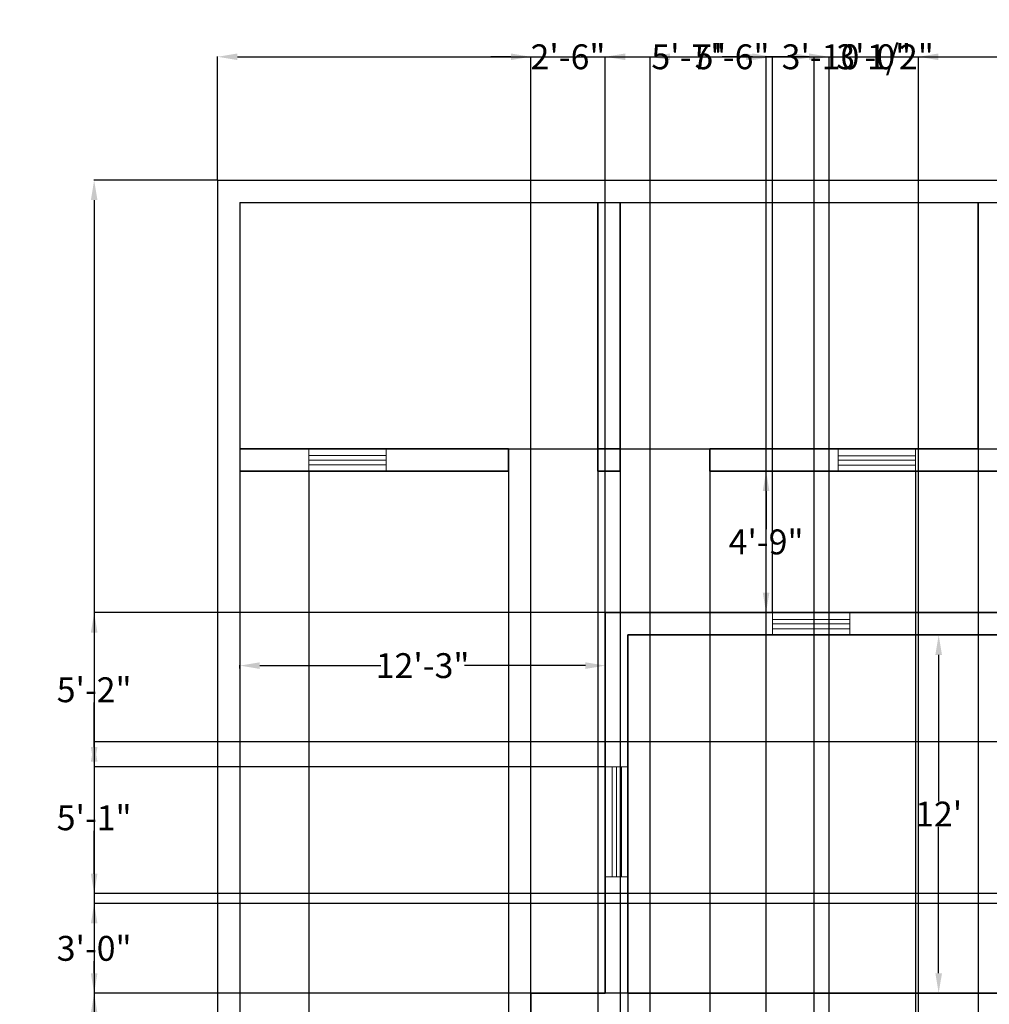
# Model space of a CAD drawing. Units: inches. Extents: x -63 to 800, y 3068 to 4133.
# Tile 4 of 5: x -63 to 327, y 3737 to 4133. Entities that reach past the tile are written whole.
import ezdxf

# ---------------------------------------------------------------- set-up
doc = ezdxf.new("R2010")
doc.units = ezdxf.units.IN
doc.header["$MEASUREMENT"] = 0
for name, color, linetype, lineweight in [('A-ANNO-DIMS', 2, 'Continuous', 13), ('A-GLAZ', 4, 'Continuous', 18), ('A-WALL', 7, 'Continuous', 35), ('A-WALL-SITE', 8, 'Continuous', 30)]:
    doc.layers.add(name, color=color, linetype=linetype, lineweight=lineweight)
doc.styles.get("Standard").update_dxf_attribs({"font": 'arial.ttf'})
doc.dimstyles.get("Standard").update_dxf_attribs({"dimtxt": 10, "dimasz": 8, "dimexe": 0.18, "dimexo": 0.0625, "dimgap": 0.09, "dimtad": 0, "dimtih": 1, "dimtoh": 1, "dimdec": 0, "dimzin": 0, "dimdsep": 46, "dimlunit": 3, "dimtxsty": 'Standard', "dimcen": 0.09, "dimadec": 0, "dimazin": 0, "dimtfac": 1, "dimtdec": 0, "dimtofl": 0, "dimtmove": 0, "dimatfit": 3, "dimfxl": 1, "dimtolj": 1, "dimtzin": 0, "dimarcsym": 0})

# ---------------------------------------------------------------- blocks, each defined once
blk = doc.blocks.new('*D2')
at = {"layer": 'A-ANNO-DIMS', "color": 0, "lineweight": -2, "transparency": 16777216}
for p, q in [((223.3, 3951.66), (237.18, 3951.66)), ((237, 3943.66), (237, 3928.43)), ((237, 3902.81), (237, 3918.04)), ((223.3, 3894.81), (237.18, 3894.81))]:
    blk.add_line(p, q, dxfattribs=at)
at = {"layer": 'A-ANNO-DIMS', "color": 0, "transparency": 16777216}
for points in [[(235.66, 3943.66), (238.33, 3943.66), (237, 3951.66)], [(235.66, 3902.81), (238.33, 3902.81), (237, 3894.81)]]:
    blk.add_solid(points, dxfattribs=at)
at = {"layer": 'Defpoints', "color": 0, "transparency": 16777216}
for p in [(223.24, 3951.66), (223.24, 3894.81), (237, 3894.81)]:
    blk.add_point(p, dxfattribs=at)
at = {"layer": 'A-ANNO-DIMS', "color": 0, "transparency": 16777216, "insert": (237, 3923.24), "char_height": 10, "attachment_point": 5}
blk.add_mtext('\\A1;4\'-9"', dxfattribs=at)
blk = doc.blocks.new('*D3')
at = {"layer": 'A-ANNO-DIMS', "color": 0, "lineweight": -2, "transparency": 16777216}
for p, q in [((25.31, 3872.29), (25.31, 3873.68)), ((33.31, 3873.5), (82.01, 3873.5)), ((164.31, 3873.5), (115.6, 3873.5)), ((172.31, 3872.29), (172.31, 3873.68))]:
    blk.add_line(p, q, dxfattribs=at)
at = {"layer": 'A-ANNO-DIMS', "color": 0, "transparency": 16777216}
for points in [[(33.31, 3874.83), (33.31, 3872.16), (25.31, 3873.5)], [(164.31, 3874.83), (164.31, 3872.16), (172.31, 3873.5)]]:
    blk.add_solid(points, dxfattribs=at)
at = {"layer": 'Defpoints', "color": 0, "transparency": 16777216}
for p in [(25.31, 3872.23), (172.31, 3873.5), (172.31, 3872.23)]:
    blk.add_point(p, dxfattribs=at)
at = {"layer": 'A-ANNO-DIMS', "color": 0, "transparency": 16777216, "insert": (98.81, 3873.5), "char_height": 10, "attachment_point": 5}
blk.add_mtext('\\A1;12\'-3"', dxfattribs=at)
blk = doc.blocks.new('*D5')
at = {"layer": 'A-ANNO-DIMS', "color": 0, "lineweight": -2, "transparency": 16777216}
for p, q in [((306.49, 3885.81), (306.61, 3885.81)), ((306.43, 3877.81), (306.43, 3818.92)), ((306.43, 3749.81), (306.43, 3808.7)), ((306.49, 3741.81), (306.61, 3741.81))]:
    blk.add_line(p, q, dxfattribs=at)
at = {"layer": 'A-ANNO-DIMS', "color": 0, "transparency": 16777216}
for points in [[(305.1, 3877.81), (307.77, 3877.81), (306.43, 3885.81)], [(305.1, 3749.81), (307.77, 3749.81), (306.43, 3741.81)]]:
    blk.add_solid(points, dxfattribs=at)
at = {"layer": 'Defpoints', "color": 0, "transparency": 16777216}
for p in [(306.43, 3885.81), (306.43, 3741.81), (306.43, 3741.81)]:
    blk.add_point(p, dxfattribs=at)
at = {"layer": 'A-ANNO-DIMS', "color": 0, "transparency": 16777216, "insert": (306.43, 3813.81), "char_height": 10, "attachment_point": 5}
blk.add_mtext("\\A1;12'", dxfattribs=at)
blk = doc.blocks.new('WIN-31')
blk.add_lwpolyline([(0, 9), (31.17, 9), (31.17, 0), (0, 0)], close=True)
blk.add_lwpolyline([(0, 4.5), (31.17, 4.5), (31.17, 6.29), (0, 6.29), (0, 2.51), (31.17, 2.51)])
blk = doc.blocks.new('WIN-44')
blk.add_lwpolyline([(0, 0), (0, 44.17), (9, 44.17), (9, 0)], close=True)
for points in [[(2.71, 44.17), (2.71, 0), (6.5, 0), (6.5, 44.17)], [(4.5, 0), (4.5, 44.17)]]:
    blk.add_lwpolyline(points)
blk = doc.blocks.new('*D19')
at = {"layer": 'A-ANNO-DIMS', "color": 0, "lineweight": -2, "transparency": 16777216}
for p, q in [((16.31, 4068.72), (16.31, 4118.49)), ((24.31, 4118.31), (351.54, 4118.31)), ((713.31, 4118.31), (386.08, 4118.31)), ((721.31, 4068.72), (721.31, 4118.49))]:
    blk.add_line(p, q, dxfattribs=at)
at = {"layer": 'A-ANNO-DIMS', "color": 0, "transparency": 16777216}
for points in [[(24.31, 4119.64), (24.31, 4116.98), (16.31, 4118.31)], [(713.31, 4119.64), (713.31, 4116.98), (721.31, 4118.31)]]:
    blk.add_solid(points, dxfattribs=at)
at = {"layer": 'Defpoints', "color": 0, "transparency": 16777216}
for p in [(721.31, 4118.31), (16.31, 4068.66), (721.31, 4068.66)]:
    blk.add_point(p, dxfattribs=at)
at = {"layer": 'A-ANNO-DIMS', "color": 0, "transparency": 16777216, "insert": (368.81, 4118.31), "char_height": 10, "attachment_point": 5}
blk.add_mtext('\\A1;58\'-9"', dxfattribs=at)
blk = doc.blocks.new('*D20')
at = {"layer": 'A-ANNO-DIMS', "color": 0, "lineweight": -2, "transparency": 16777216}
for p, q in [((16.25, 4068.66), (-33.52, 4068.66)), ((-33.34, 4060.66), (-33.34, 3605.75)), ((-33.34, 3140.31), (-33.34, 3595.23)), ((16.25, 3132.31), (-33.52, 3132.31))]:
    blk.add_line(p, q, dxfattribs=at)
at = {"layer": 'A-ANNO-DIMS', "color": 0, "transparency": 16777216}
for points in [[(-34.67, 4060.66), (-32.01, 4060.66), (-33.34, 4068.66)], [(-34.67, 3140.31), (-32.01, 3140.31), (-33.34, 3132.31)]]:
    blk.add_solid(points, dxfattribs=at)
at = {"layer": 'Defpoints', "color": 0, "transparency": 16777216}
for p in [(-33.34, 4068.66), (16.31, 4068.66), (16.31, 3132.31)]:
    blk.add_point(p, dxfattribs=at)
at = {"layer": 'A-ANNO-DIMS', "color": 0, "transparency": 16777216, "insert": (-33.34, 3600.49), "char_height": 10, "attachment_point": 5}
blk.add_mtext('\\A1;78\'-0 1/2"', dxfattribs=at)
blk = doc.blocks.new('*D23')
at = {"layer": 'A-ANNO-DIMS', "color": 0, "lineweight": -2, "transparency": 16777216}
for p, q in [((25.31, 4059.6), (25.31, 3082.48)), ((169.31, 4059.6), (169.31, 3082.48)), ((33.31, 3082.66), (80.51, 3082.66)), ((161.31, 3082.66), (114.1, 3082.66))]:
    blk.add_line(p, q, dxfattribs=at)
at = {"layer": 'A-ANNO-DIMS', "color": 0, "transparency": 16777216}
for points in [[(33.31, 3083.99), (33.31, 3081.33), (25.31, 3082.66)], [(161.31, 3083.99), (161.31, 3081.33), (169.31, 3082.66)]]:
    blk.add_solid(points, dxfattribs=at)
at = {"layer": 'Defpoints', "color": 0, "transparency": 16777216}
for p in [(25.31, 4059.66), (169.31, 4059.66), (169.31, 3082.66)]:
    blk.add_point(p, dxfattribs=at)
at = {"layer": 'A-ANNO-DIMS', "color": 0, "transparency": 16777216, "insert": (97.31, 3082.66), "char_height": 10, "attachment_point": 5}
blk.add_mtext('\\A1;12\'-0"', dxfattribs=at)
blk = doc.blocks.new('*D24')
at = {"layer": 'A-ANNO-DIMS', "color": 0, "lineweight": -2, "transparency": 16777216}
for p, q in [((178.31, 4059.6), (178.31, 3082.48)), ((322.31, 4059.6), (322.31, 3082.48)), ((186.31, 3082.66), (233.51, 3082.66)), ((314.31, 3082.66), (267.1, 3082.66))]:
    blk.add_line(p, q, dxfattribs=at)
at = {"layer": 'A-ANNO-DIMS', "color": 0, "transparency": 16777216}
for points in [[(186.31, 3083.99), (186.31, 3081.33), (178.31, 3082.66)], [(314.31, 3083.99), (314.31, 3081.33), (322.31, 3082.66)]]:
    blk.add_solid(points, dxfattribs=at)
at = {"layer": 'Defpoints', "color": 0, "transparency": 16777216}
for p in [(178.31, 4059.66), (322.31, 4059.66), (322.31, 3082.66)]:
    blk.add_point(p, dxfattribs=at)
at = {"layer": 'A-ANNO-DIMS', "color": 0, "transparency": 16777216, "insert": (250.31, 3082.66), "char_height": 10, "attachment_point": 5}
blk.add_mtext('\\A1;12\'-0"', dxfattribs=at)
blk = doc.blocks.new('*D26')
at = {"layer": 'A-ANNO-DIMS', "color": 0, "lineweight": -2, "transparency": 16777216}
for p, q in [((25.37, 4059.66), (771.14, 4059.66)), ((770.96, 4051.66), (770.96, 4015.36)), ((770.96, 3968.66), (770.96, 4004.96)), ((25.37, 3960.66), (771.14, 3960.66))]:
    blk.add_line(p, q, dxfattribs=at)
at = {"layer": 'A-ANNO-DIMS', "color": 0, "transparency": 16777216}
for points in [[(769.63, 4051.66), (772.29, 4051.66), (770.96, 4059.66)], [(769.63, 3968.66), (772.29, 3968.66), (770.96, 3960.66)]]:
    blk.add_solid(points, dxfattribs=at)
at = {"layer": 'Defpoints', "color": 0, "transparency": 16777216}
for p in [(25.31, 4059.66), (770.96, 4059.66), (25.31, 3960.66)]:
    blk.add_point(p, dxfattribs=at)
at = {"layer": 'A-ANNO-DIMS', "color": 0, "transparency": 16777216, "insert": (770.96, 4010.16), "char_height": 10, "attachment_point": 5}
blk.add_mtext('\\A1;8\'-3"', dxfattribs=at)
blk = doc.blocks.new('*D27')
at = {"layer": 'A-ANNO-DIMS', "color": 0, "lineweight": -2, "transparency": 16777216}
for p, q in [((25.31, 3951.6), (25.31, 3082.48)), ((52.97, 3951.6), (52.97, 3082.48)), ((33.31, 3082.66), (44.97, 3082.66)), ((52.97, 3082.66), (60.97, 3082.66))]:
    blk.add_line(p, q, dxfattribs=at)
at = {"layer": 'A-ANNO-DIMS', "color": 0, "transparency": 16777216}
for points in [[(33.31, 3083.99), (33.31, 3081.33), (25.31, 3082.66)], [(44.97, 3083.99), (44.97, 3081.33), (52.97, 3082.66)]]:
    blk.add_solid(points, dxfattribs=at)
at = {"layer": 'Defpoints', "color": 0, "transparency": 16777216}
for p in [(25.31, 3951.66), (52.97, 3951.66), (52.97, 3082.66)]:
    blk.add_point(p, dxfattribs=at)
at = {"layer": 'A-ANNO-DIMS', "color": 0, "transparency": 16777216, "insert": (86.08, 3082.66), "char_height": 10, "attachment_point": 5}
blk.add_mtext('\\A1;2\'-3 1/2"', dxfattribs=at)
blk = doc.blocks.new('*D28')
at = {"layer": 'A-ANNO-DIMS', "color": 0, "lineweight": -2, "transparency": 16777216}
for p, q in [((297.16, 3951.55), (297.16, 3082.48)), ((331.31, 3951.6), (331.31, 3082.48)), ((305.16, 3082.66), (323.31, 3082.66)), ((331.31, 3082.66), (339.31, 3082.66))]:
    blk.add_line(p, q, dxfattribs=at)
at = {"layer": 'A-ANNO-DIMS', "color": 0, "transparency": 16777216}
for points in [[(305.16, 3083.99), (305.16, 3081.33), (297.16, 3082.66)], [(323.31, 3083.99), (323.31, 3081.33), (331.31, 3082.66)]]:
    blk.add_solid(points, dxfattribs=at)
at = {"layer": 'Defpoints', "color": 0, "transparency": 16777216}
for p in [(297.16, 3951.61), (331.31, 3951.66), (331.31, 3082.66)]:
    blk.add_point(p, dxfattribs=at)
at = {"layer": 'A-ANNO-DIMS', "color": 0, "transparency": 16777216, "insert": (356.66, 3082.66), "char_height": 10, "attachment_point": 5}
blk.add_mtext('\\A1;2\'-10"', dxfattribs=at)
blk = doc.blocks.new('*D30')
at = {"layer": 'A-ANNO-DIMS', "color": 0, "lineweight": -2, "transparency": 16777216}
for p, q in [((133.31, 3951.6), (133.31, 3082.48)), ((169.31, 3951.6), (169.31, 3082.48)), ((125.31, 3082.66), (117.31, 3082.66)), ((177.31, 3082.66), (185.31, 3082.66))]:
    blk.add_line(p, q, dxfattribs=at)
at = {"layer": 'A-ANNO-DIMS', "color": 0, "transparency": 16777216}
for points in [[(125.31, 3083.99), (125.31, 3081.33), (133.31, 3082.66)], [(177.31, 3083.99), (177.31, 3081.33), (169.31, 3082.66)]]:
    blk.add_solid(points, dxfattribs=at)
at = {"layer": 'Defpoints', "color": 0, "transparency": 16777216}
for p in [(133.31, 3951.66), (169.31, 3951.66), (169.31, 3082.66)]:
    blk.add_point(p, dxfattribs=at)
at = {"layer": 'A-ANNO-DIMS', "color": 0, "transparency": 16777216, "insert": (151.31, 3082.66), "char_height": 10, "attachment_point": 5}
blk.add_mtext('\\A1;3\'-0"', dxfattribs=at)
blk = doc.blocks.new('*D31')
at = {"layer": 'A-ANNO-DIMS', "color": 0, "lineweight": -2, "transparency": 16777216}
for p, q in [((178.31, 3951.6), (178.31, 3082.48)), ((214.31, 3951.6), (214.31, 3082.48)), ((170.31, 3082.66), (162.31, 3082.66)), ((222.31, 3082.66), (230.31, 3082.66))]:
    blk.add_line(p, q, dxfattribs=at)
at = {"layer": 'A-ANNO-DIMS', "color": 0, "transparency": 16777216}
for points in [[(170.31, 3083.99), (170.31, 3081.33), (178.31, 3082.66)], [(222.31, 3083.99), (222.31, 3081.33), (214.31, 3082.66)]]:
    blk.add_solid(points, dxfattribs=at)
at = {"layer": 'Defpoints', "color": 0, "transparency": 16777216}
for p in [(178.31, 3951.66), (214.31, 3951.66), (214.31, 3082.66)]:
    blk.add_point(p, dxfattribs=at)
at = {"layer": 'A-ANNO-DIMS', "color": 0, "transparency": 16777216, "insert": (196.31, 3082.66), "char_height": 10, "attachment_point": 5}
blk.add_mtext('\\A1;3\'-0"', dxfattribs=at)
blk = doc.blocks.new('*D32')
at = {"layer": 'A-ANNO-DIMS', "color": 0, "lineweight": -2, "transparency": 16777216}
for p, q in [((331.31, 3951.6), (331.31, 3082.48)), ((367.31, 3951.6), (367.31, 3082.48)), ((323.31, 3082.66), (315.31, 3082.66)), ((375.31, 3082.66), (383.31, 3082.66))]:
    blk.add_line(p, q, dxfattribs=at)
at = {"layer": 'A-ANNO-DIMS', "color": 0, "transparency": 16777216}
for points in [[(323.31, 3083.99), (323.31, 3081.33), (331.31, 3082.66)], [(375.31, 3083.99), (375.31, 3081.33), (367.31, 3082.66)]]:
    blk.add_solid(points, dxfattribs=at)
at = {"layer": 'Defpoints', "color": 0, "transparency": 16777216}
for p in [(331.31, 3951.66), (367.31, 3951.66), (367.31, 3082.66)]:
    blk.add_point(p, dxfattribs=at)
at = {"layer": 'A-ANNO-DIMS', "color": 0, "transparency": 16777216, "insert": (349.31, 3082.66), "char_height": 10, "attachment_point": 5}
blk.add_mtext('\\A1;3\'-0"', dxfattribs=at)
blk = doc.blocks.new('*D36')
at = {"layer": 'A-ANNO-DIMS', "color": 0, "lineweight": -2, "transparency": 16777216}
for p, q in [((134.31, 4118.31), (126.31, 4118.31)), ((142.31, 3741.87), (142.31, 4118.49)), ((172.31, 3741.87), (172.31, 4118.49)), ((180.31, 4118.31), (188.31, 4118.31))]:
    blk.add_line(p, q, dxfattribs=at)
at = {"layer": 'A-ANNO-DIMS', "color": 0, "transparency": 16777216}
for points in [[(134.31, 4119.64), (134.31, 4116.98), (142.31, 4118.31)], [(180.31, 4119.64), (180.31, 4116.98), (172.31, 4118.31)]]:
    blk.add_solid(points, dxfattribs=at)
at = {"layer": 'Defpoints', "color": 0, "transparency": 16777216}
for p in [(172.31, 4118.31), (142.31, 3741.81), (172.31, 3741.81)]:
    blk.add_point(p, dxfattribs=at)
at = {"layer": 'A-ANNO-DIMS', "color": 0, "transparency": 16777216, "insert": (157.31, 4118.31), "char_height": 10, "attachment_point": 5}
blk.add_mtext('\\A1;2\'-6"', dxfattribs=at)
blk = doc.blocks.new('*D37')
at = {"layer": 'A-ANNO-DIMS', "color": 0, "lineweight": -2, "transparency": 16777216}
for p, q in [((181.31, 3885.75), (181.31, 3082.48)), ((349.31, 3885.75), (349.31, 3082.48)), ((189.31, 3082.66), (248.51, 3082.66)), ((341.31, 3082.66), (282.1, 3082.66))]:
    blk.add_line(p, q, dxfattribs=at)
at = {"layer": 'A-ANNO-DIMS', "color": 0, "transparency": 16777216}
for points in [[(189.31, 3083.99), (189.31, 3081.33), (181.31, 3082.66)], [(341.31, 3083.99), (341.31, 3081.33), (349.31, 3082.66)]]:
    blk.add_solid(points, dxfattribs=at)
at = {"layer": 'Defpoints', "color": 0, "transparency": 16777216}
for p in [(181.31, 3885.81), (349.31, 3885.81), (349.31, 3082.66)]:
    blk.add_point(p, dxfattribs=at)
at = {"layer": 'A-ANNO-DIMS', "color": 0, "transparency": 16777216, "insert": (265.31, 3082.66), "char_height": 10, "attachment_point": 5}
blk.add_mtext('\\A1;14\'-0"', dxfattribs=at)
blk = doc.blocks.new('*D40')
at = {"layer": 'A-ANNO-DIMS', "color": 0, "lineweight": -2, "transparency": 16777216}
for p, q in [((172.31, 3894.87), (172.31, 4118.49)), ((180.31, 4118.31), (192.53, 4118.31)), ((231.52, 4118.31), (219.29, 4118.31)), ((239.52, 3894.87), (239.52, 4118.49))]:
    blk.add_line(p, q, dxfattribs=at)
at = {"layer": 'A-ANNO-DIMS', "color": 0, "transparency": 16777216}
for points in [[(180.31, 4119.64), (180.31, 4116.98), (172.31, 4118.31)], [(231.52, 4119.64), (231.52, 4116.98), (239.52, 4118.31)]]:
    blk.add_solid(points, dxfattribs=at)
at = {"layer": 'Defpoints', "color": 0, "transparency": 16777216}
for p in [(239.52, 4118.31), (172.31, 3894.81), (239.52, 3894.81)]:
    blk.add_point(p, dxfattribs=at)
at = {"layer": 'A-ANNO-DIMS', "color": 0, "transparency": 16777216, "insert": (205.91, 4118.31), "char_height": 10, "attachment_point": 5}
blk.add_mtext('\\A1;5\'-7"', dxfattribs=at)
blk = doc.blocks.new('*D42')
at = {"layer": 'A-ANNO-DIMS', "color": 0, "lineweight": -2, "transparency": 16777216}
for p, q in [((172.25, 3894.81), (-33.52, 3894.81)), ((-33.34, 3886.81), (-33.34, 3868.99)), ((-33.34, 3840.77), (-33.34, 3858.6)), ((172.25, 3832.77), (-33.52, 3832.77))]:
    blk.add_line(p, q, dxfattribs=at)
at = {"layer": 'A-ANNO-DIMS', "color": 0, "transparency": 16777216}
for points in [[(-34.67, 3886.81), (-32.01, 3886.81), (-33.34, 3894.81)], [(-34.67, 3840.77), (-32.01, 3840.77), (-33.34, 3832.77)]]:
    blk.add_solid(points, dxfattribs=at)
at = {"layer": 'Defpoints', "color": 0, "transparency": 16777216}
for p in [(-33.34, 3894.81), (172.31, 3894.81), (172.31, 3832.77)]:
    blk.add_point(p, dxfattribs=at)
at = {"layer": 'A-ANNO-DIMS', "color": 0, "transparency": 16777216, "insert": (-33.34, 3863.79), "char_height": 10, "attachment_point": 5}
blk.add_mtext('\\A1;5\'-2"', dxfattribs=at)
blk = doc.blocks.new('*D49')
at = {"layer": 'A-ANNO-DIMS', "color": 0, "lineweight": -2, "transparency": 16777216}
for p, q in [((142.25, 3741.81), (-33.52, 3741.81)), ((-33.34, 3733.81), (-33.34, 3716.81)), ((-33.34, 3689.29), (-33.34, 3706.29)), ((142.25, 3681.29), (-33.52, 3681.29))]:
    blk.add_line(p, q, dxfattribs=at)
at = {"layer": 'A-ANNO-DIMS', "color": 0, "transparency": 16777216}
for points in [[(-34.67, 3733.81), (-32.01, 3733.81), (-33.34, 3741.81)], [(-34.67, 3689.29), (-32.01, 3689.29), (-33.34, 3681.29)]]:
    blk.add_solid(points, dxfattribs=at)
at = {"layer": 'Defpoints', "color": 0, "transparency": 16777216}
for p in [(-33.34, 3741.81), (142.31, 3741.81), (142.31, 3681.29)]:
    blk.add_point(p, dxfattribs=at)
at = {"layer": 'A-ANNO-DIMS', "color": 0, "transparency": 16777216, "insert": (-33.34, 3711.55), "char_height": 10, "attachment_point": 5}
blk.add_mtext('\\A1;5\'-0 1/2"', dxfattribs=at)
blk = doc.blocks.new('*D57')
at = {"layer": 'A-ANNO-DIMS', "color": 0, "lineweight": -2, "transparency": 16777216}
for p, q in [((190.31, 3311.37), (190.31, 4118.49)), ((198.31, 4118.31), (228.97, 4118.31)), ((236.97, 3320.37), (236.97, 4118.49)), ((236.97, 4118.31), (244.97, 4118.31))]:
    blk.add_line(p, q, dxfattribs=at)
at = {"layer": 'A-ANNO-DIMS', "color": 0, "transparency": 16777216}
for points in [[(198.31, 4119.64), (198.31, 4116.98), (190.31, 4118.31)], [(228.97, 4119.64), (228.97, 4116.98), (236.97, 4118.31)]]:
    blk.add_solid(points, dxfattribs=at)
at = {"layer": 'Defpoints', "color": 0, "transparency": 16777216}
for p in [(236.97, 4118.31), (236.97, 3320.31), (190.31, 3311.31)]:
    blk.add_point(p, dxfattribs=at)
at = {"layer": 'A-ANNO-DIMS', "color": 0, "transparency": 16777216, "insert": (273.88, 4118.31), "char_height": 10, "attachment_point": 5}
blk.add_mtext('\\A1;3\'-10 1/2"', dxfattribs=at)
blk = doc.blocks.new('*D64')
at = {"layer": 'A-ANNO-DIMS', "color": 0, "lineweight": -2, "transparency": 16777216}
for p, q in [((190.31, 3473.37), (190.31, 4118.49)), ((198.31, 4118.31), (209.93, 4118.31)), ((248.31, 4118.31), (236.69, 4118.31)), ((256.31, 3473.37), (256.31, 4118.49))]:
    blk.add_line(p, q, dxfattribs=at)
at = {"layer": 'A-ANNO-DIMS', "color": 0, "transparency": 16777216}
for points in [[(198.31, 4119.64), (198.31, 4116.98), (190.31, 4118.31)], [(248.31, 4119.64), (248.31, 4116.98), (256.31, 4118.31)]]:
    blk.add_solid(points, dxfattribs=at)
at = {"layer": 'Defpoints', "color": 0, "transparency": 16777216}
for p in [(256.31, 4118.31), (190.31, 3473.31), (256.31, 3473.31)]:
    blk.add_point(p, dxfattribs=at)
at = {"layer": 'A-ANNO-DIMS', "color": 0, "transparency": 16777216, "insert": (223.31, 4118.31), "char_height": 10, "attachment_point": 5}
blk.add_mtext('\\A1;5\'-6"', dxfattribs=at)
blk = doc.blocks.new('*D66')
at = {"layer": 'A-ANNO-DIMS', "color": 0, "lineweight": -2, "transparency": 16777216}
for p, q in [((378.25, 3842.81), (-33.52, 3842.81)), ((-33.34, 3834.81), (-33.34, 3817.51)), ((-33.34, 3789.81), (-33.34, 3807.11)), ((378.25, 3781.81), (-33.52, 3781.81))]:
    blk.add_line(p, q, dxfattribs=at)
at = {"layer": 'A-ANNO-DIMS', "color": 0, "transparency": 16777216}
for points in [[(-34.67, 3834.81), (-32.01, 3834.81), (-33.34, 3842.81)], [(-34.67, 3789.81), (-32.01, 3789.81), (-33.34, 3781.81)]]:
    blk.add_solid(points, dxfattribs=at)
at = {"layer": 'Defpoints', "color": 0, "transparency": 16777216}
for p in [(-33.34, 3842.81), (378.31, 3842.81), (378.31, 3781.81)]:
    blk.add_point(p, dxfattribs=at)
at = {"layer": 'A-ANNO-DIMS', "color": 0, "transparency": 16777216, "insert": (-33.34, 3812.31), "char_height": 10, "attachment_point": 5}
blk.add_mtext('\\A1;5\'-1"', dxfattribs=at)
blk = doc.blocks.new('*D67')
at = {"layer": 'A-ANNO-DIMS', "color": 0, "lineweight": -2, "transparency": 16777216}
for p, q in [((505.25, 3777.81), (-33.52, 3777.81)), ((-33.34, 3769.81), (-33.34, 3765.01)), ((-33.34, 3749.81), (-33.34, 3754.61)), ((631.25, 3741.81), (-33.52, 3741.81))]:
    blk.add_line(p, q, dxfattribs=at)
at = {"layer": 'A-ANNO-DIMS', "color": 0, "transparency": 16777216}
for points in [[(-34.67, 3769.81), (-32.01, 3769.81), (-33.34, 3777.81)], [(-34.67, 3749.81), (-32.01, 3749.81), (-33.34, 3741.81)]]:
    blk.add_solid(points, dxfattribs=at)
at = {"layer": 'Defpoints', "color": 0, "transparency": 16777216}
for p in [(505.31, 3777.81), (-33.34, 3741.81), (631.31, 3741.81)]:
    blk.add_point(p, dxfattribs=at)
at = {"layer": 'A-ANNO-DIMS', "color": 0, "transparency": 16777216, "insert": (-33.34, 3759.81), "char_height": 10, "attachment_point": 5}
blk.add_mtext('\\A1;3\'-0"', dxfattribs=at)
blk = doc.blocks.new('*D68')
at = {"layer": 'A-ANNO-DIMS', "color": 0, "lineweight": -2, "transparency": 16777216}
for p, q in [((254.31, 4118.31), (246.31, 4118.31)), ((262.31, 3594.87), (262.31, 4118.49)), ((298.31, 3549.87), (298.31, 4118.49)), ((306.31, 4118.31), (314.31, 4118.31))]:
    blk.add_line(p, q, dxfattribs=at)
at = {"layer": 'A-ANNO-DIMS', "color": 0, "transparency": 16777216}
for points in [[(254.31, 4119.64), (254.31, 4116.98), (262.31, 4118.31)], [(306.31, 4119.64), (306.31, 4116.98), (298.31, 4118.31)]]:
    blk.add_solid(points, dxfattribs=at)
at = {"layer": 'Defpoints', "color": 0, "transparency": 16777216}
for p in [(298.31, 4118.31), (262.31, 3594.81), (298.31, 3549.81)]:
    blk.add_point(p, dxfattribs=at)
at = {"layer": 'A-ANNO-DIMS', "color": 0, "transparency": 16777216, "insert": (280.31, 4118.31), "char_height": 10, "attachment_point": 5}
blk.add_mtext('\\A1;3\'-0"', dxfattribs=at)

msp = doc.modelspace()

# ---------------------------------------------------------------- linework, layer by layer
at = {"layer": 'A-WALL'}
for p, q in [((169.31, 4059.66), (169.31, 3951.66)), ((178.31, 4059.66), (178.31, 3951.66)), ((322.31, 4059.66), (322.31, 3960.66)), ((25.31, 3960.66), (133.31, 3960.66)), ((169.31, 3960.66), (178.31, 3960.66)), ((214.31, 3960.66), (322.31, 3960.66)), ((25.31, 3951.66), (133.31, 3951.66)), ((169.31, 3951.66), (178.31, 3951.66)), ((214.31, 3951.66), (331.31, 3951.66)), ((172.31, 3894.81), (640.31, 3894.81)), ((172.31, 3894.81), (172.31, 3741.81)), ((181.31, 3885.81), (349.31, 3885.81)), ((181.31, 3885.81), (181.31, 3741.81)), ((181.31, 3885.81), (181.31, 3741.81)), ((142.31, 3741.81), (172.31, 3741.81)), ((142.31, 3741.81), (142.31, 3522.81)), ((181.31, 3741.81), (496.31, 3741.81))]:
    msp.add_line(p, q, dxfattribs=at)
for points in [[(133.31, 3951.66), (133.31, 3960.66)], [(169.31, 3960.66), (169.31, 3951.66)], [(178.31, 3951.66), (178.31, 3960.66)], [(214.31, 3960.66), (214.31, 3951.66)]]:
    msp.add_lwpolyline(points, dxfattribs=at)
at = {"layer": 'A-WALL-SITE'}
for p, q in [((16.31, 4068.66), (16.31, 3132.31)), ((16.31, 4068.66), (721.31, 4068.66)), ((25.31, 4059.66), (25.31, 3960.66)), ((25.31, 4059.66), (169.31, 4059.66)), ((178.31, 4059.66), (322.31, 4059.66)), ((25.31, 3951.66), (25.31, 3132.31))]:
    msp.add_line(p, q, dxfattribs=at)

# ---------------------------------------------------------------- block references
at = {"layer": 'A-GLAZ'}
for name, p in [('WIN-31', (52.97, 3951.66)), ('WIN-31', (265.99, 3951.61)), ('WIN-31', (239.52, 3885.81)), ('WIN-44', (172.31, 3788.6))]:
    msp.add_blockref(name, p, dxfattribs=at)

# ---------------------------------------------------------------- dimensions: what is measured, and where the dimension line sits
at = {"layer": 'A-ANNO-DIMS'}
for base, p1, p2, override, picture, middle in [((236.97, 4118.31), (190.31, 3311.31), (236.97, 3320.31), {"dimdec": 1, "dimlfac": 1, "dimrnd": 0, "dimzin": 1, "dimdsep": 46, "dimlunit": 4, "dimfrac": 2}, '*D57', (273.88, 4118.31)), ((721.31, 4118.31), (16.31, 4068.66), (721.31, 4068.66), {"dimdec": 1, "dimlfac": 1, "dimrnd": 0, "dimzin": 1, "dimdsep": 46, "dimlunit": 4, "dimfrac": 2}, '*D19', (368.81, 4118.31)), ((172.31, 4118.31), (142.31, 3741.81), (172.31, 3741.81), {"dimdec": 1, "dimlfac": 1, "dimrnd": 0, "dimzin": 1, "dimdsep": 46, "dimlunit": 4, "dimfrac": 2}, '*D36', (157.31, 4118.31)), ((239.52, 4118.31), (172.31, 3894.81), (239.52, 3894.81), {"dimdec": 1, "dimlfac": 1, "dimrnd": 0, "dimzin": 1, "dimdsep": 46, "dimlunit": 4, "dimfrac": 2}, '*D40', (205.91, 4118.31)), ((256.31, 4118.31), (190.31, 3473.31), (256.31, 3473.31), {"dimdec": 1, "dimlfac": 1, "dimrnd": 0, "dimzin": 1, "dimdsep": 46, "dimlunit": 4, "dimfrac": 2}, '*D64', (223.31, 4118.31)), ((298.31, 4118.31), (262.31, 3594.81), (298.31, 3549.81), {"dimdec": 1, "dimlfac": 1, "dimrnd": 0, "dimzin": 1, "dimdsep": 46, "dimlunit": 4, "dimfrac": 2}, '*D68', (280.31, 4118.31)), ((169.31, 3082.66), (25.31, 4059.66), (169.31, 4059.66), {"dimdec": 1, "dimlfac": 1, "dimrnd": 0, "dimzin": 1, "dimdsep": 46, "dimlunit": 4, "dimfrac": 2}, '*D23', (97.31, 3082.66)), ((322.31, 3082.66), (178.31, 4059.66), (322.31, 4059.66), {"dimdec": 1, "dimlfac": 1, "dimrnd": 0, "dimzin": 1, "dimdsep": 46, "dimlunit": 4, "dimfrac": 2}, '*D24', (250.31, 3082.66)), ((52.97, 3082.66), (25.31, 3951.66), (52.97, 3951.66), {"dimdec": 1, "dimlfac": 1, "dimrnd": 0, "dimzin": 1, "dimdsep": 46, "dimlunit": 4, "dimfrac": 2}, '*D27', (86.08, 3082.66)), ((169.31, 3082.66), (133.31, 3951.66), (169.31, 3951.66), {"dimdec": 1, "dimlfac": 1, "dimrnd": 0, "dimzin": 1, "dimdsep": 46, "dimlunit": 4, "dimfrac": 2}, '*D30', (151.31, 3082.66)), ((214.31, 3082.66), (178.31, 3951.66), (214.31, 3951.66), {"dimdec": 1, "dimlfac": 1, "dimrnd": 0, "dimzin": 1, "dimdsep": 46, "dimlunit": 4, "dimfrac": 2}, '*D31', (196.31, 3082.66)), ((331.3095, 3082.6602), (297.1617, 3951.6131), (331.3095, 3951.6613), {"dimdec": 1, "dimlfac": 1, "dimrnd": 0, "dimzin": 1, "dimdsep": 46, "dimlunit": 4, "dimfrac": 2}, '*D28', (356.6607, 3082.6602)), ((367.31, 3082.66), (331.31, 3951.66), (367.31, 3951.66), {"dimdec": 1, "dimlfac": 1, "dimrnd": 0, "dimzin": 1, "dimdsep": 46, "dimlunit": 4, "dimfrac": 2}, '*D32', (349.31, 3082.66)), ((349.31, 3082.66), (181.31, 3885.81), (349.31, 3885.81), {"dimdec": 1, "dimlfac": 1, "dimrnd": 0, "dimzin": 1, "dimdsep": 46, "dimlunit": 4, "dimfrac": 2}, '*D37', (265.31, 3082.66)), ((172.31, 3873.5), (25.31, 3872.23), (172.31, 3872.23), {"dimclrd": 0, "dimclre": 0, "dimclrt": 0}, '*D3', (98.81, 3873.5))]:
    dim = msp.add_linear_dim(base=base, p1=p1, p2=p2, dimstyle='Standard', override=override, dxfattribs=at)
    dim.commit()
    dim.dimension.update_dxf_attribs({"geometry": picture, "text_midpoint": middle})
for base, p1, p2, override, picture, middle in [((-33.3405, 4068.6613), (16.3095, 3132.3102), (16.3095, 4068.6613), {"dimdec": 1, "dimlfac": 1, "dimrnd": 0, "dimzin": 1, "dimdsep": 46, "dimlunit": 4, "dimfrac": 2}, '*D20', (-33.3405, 3600.4858)), ((770.96, 4059.66), (25.31, 3960.66), (25.31, 4059.66), {"dimdec": 1, "dimlfac": 1, "dimrnd": 0, "dimzin": 1, "dimdsep": 46, "dimlunit": 4, "dimfrac": 2}, '*D26', (770.96, 4010.16)), ((237, 3894.81), (223.24, 3951.66), (223.24, 3894.81), {"dimclrd": 0, "dimclre": 0, "dimclrt": 0}, '*D2', (237, 3923.24)), ((-33.34, 3894.81), (172.31, 3832.77), (172.31, 3894.81), {"dimdec": 1, "dimlfac": 1, "dimrnd": 0, "dimzin": 1, "dimdsep": 46, "dimlunit": 4, "dimfrac": 2}, '*D42', (-33.34, 3863.79)), ((306.43, 3741.81), (306.43, 3885.81), (306.43, 3741.81), {"dimclrd": 0, "dimclre": 0, "dimclrt": 0}, '*D5', (306.43, 3813.81)), ((-33.34, 3842.81), (378.31, 3781.81), (378.31, 3842.81), {"dimdec": 1, "dimlfac": 1, "dimrnd": 0, "dimzin": 1, "dimdsep": 46, "dimlunit": 4, "dimfrac": 2}, '*D66', (-33.34, 3812.31)), ((-33.34, 3741.81), (505.31, 3777.81), (631.31, 3741.81), {"dimdec": 1, "dimlfac": 1, "dimrnd": 0, "dimzin": 1, "dimdsep": 46, "dimlunit": 4, "dimfrac": 2}, '*D67', (-33.34, 3759.81)), ((-33.34, 3741.81), (142.31, 3681.29), (142.31, 3741.81), {"dimdec": 1, "dimlfac": 1, "dimrnd": 0, "dimzin": 1, "dimdsep": 46, "dimlunit": 4, "dimfrac": 2}, '*D49', (-33.34, 3711.55))]:
    dim = msp.add_linear_dim(base=base, p1=p1, p2=p2, angle=90, dimstyle='Standard', override=override, dxfattribs=at)
    dim.commit()
    dim.dimension.update_dxf_attribs({"geometry": picture, "text_midpoint": middle})

doc.saveas('drawing.dxf')
